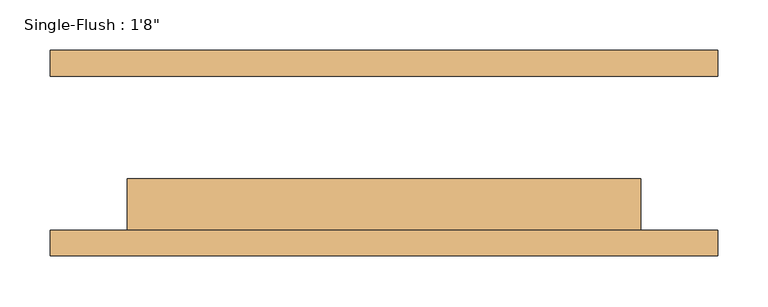
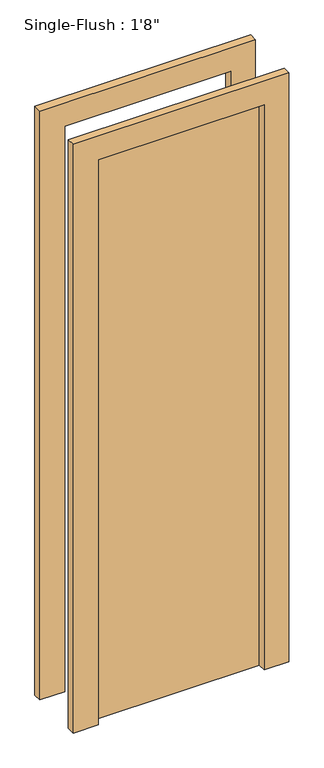
"""IFC4 building model written with IfcOpenShell, lengths in millimetres: door geometry."""

from ifc_helpers import new_model, si_unit, frame, origin, origin_with_axes, place, context, project, spatial, polyline, outline, extrude, source, transform, mapped, element, save


def door_85c31a06(model_context):
    return source(origin(), model_context, "Body", "SweptSolid", [
        extrude(outline(polyline([(1905.0, -330.2), (0.0, -330.2), (0.0, -254.0), (1828.8, -254.0), (1828.8, 254.0), (0.0, 254.0), (0.0, 330.2), (1905.0, 330.2), (1905.0, -330.2)])), frame((0.0, -101.6, 0.0), z_axis=(0.0, 1.0, 0.0), x_axis=(0.0, 0.0, 1.0)), (0.0, 0.0, 1.0), 25.4),
        extrude(outline(polyline([(1905.0, 330.2), (1905.0, -330.2), (0.0, -330.2), (0.0, -254.0), (1828.8, -254.0), (1828.8, 254.0), (0.0, 254.0), (0.0, 330.2), (1905.0, 330.2)])), frame((0.0, 76.2, 0.0), z_axis=(0.0, 1.0, 0.0), x_axis=(0.0, 0.0, 1.0)), (0.0, 0.0, 1.0), 25.4),
        extrude(outline(polyline([(254.0, -25.4), (254.0, -76.2), (-254.0, -76.2), (-254.0, -25.4), (254.0, -25.4)])), origin_with_axes(), (0.0, 0.0, 1.0), 1828.8),
    ])


if __name__ == "__main__":
    model = new_model("IFC4")
    model_context = context("Model", 3, world=origin())
    ifc_project = project(units=[si_unit("LENGTHUNIT", "METRE", prefix="MILLI")], contexts=[model_context])
    site = spatial("IfcSite", under=ifc_project)
    building = spatial("IfcBuilding", under=site)
    placement = place(None, origin())
    door_shape = door_85c31a06(model_context)
    element("IfcDoor", 1, ObjectType="Single-Flush : 1'8\"", at=placement, inside=building, context=model_context, shape_type="MappedRepresentation", body=[
        mapped(door_shape, transform((0.0, 0.0, 0.0), x_axis=(1.0, 0.0, 0.0), y_axis=(0.0, 1.0, 0.0), z_axis=(0.0, 0.0, 1.0))),
    ])
    save(model, "model.ifc")

# Revit data of these elements
# Type "Single-Flush : 1'8\""
#   Type Mark = "11"
#   Construction Type Id = "MDOOR"
#   Assembly Code = "C1020"
#   Analytic Construction = "Metal"
#   Thickness = 0' - 2"
#   Heat Transfer Coefficient (U) = 0.651978 BTU/(h·ft²·°F)
#   Height = 6' - 0"
#   Trim Projection Ext = 0' - 1"
#   Trim Projection Int = 0' - 1"
#   Trim Width = 0' - 3"
#   Width = 1' - 8"
#   Define Thermal Properties by = 1
#   Door Material = Door - Panel
#   Frame Material = Door - Frame
#   Visual Light Transmittance = 0
#   Solar Heat Gain Coefficient = 0
#   Function = (empty or 0)
#   Wall Closure = (empty or 0)
# Element 1 (IfcDoor, "Single-Flush : 1'8\"")
#   Materials on its faces: "Door - Frame", "Door - Panel"
# Materials
#   "Door - Panel": class "Wood", colour RGB 210 159 95, transparency 0, Cost = 0
#   "Door - Frame": colour RGB 118 70 51, transparency 0, Cost = 0
